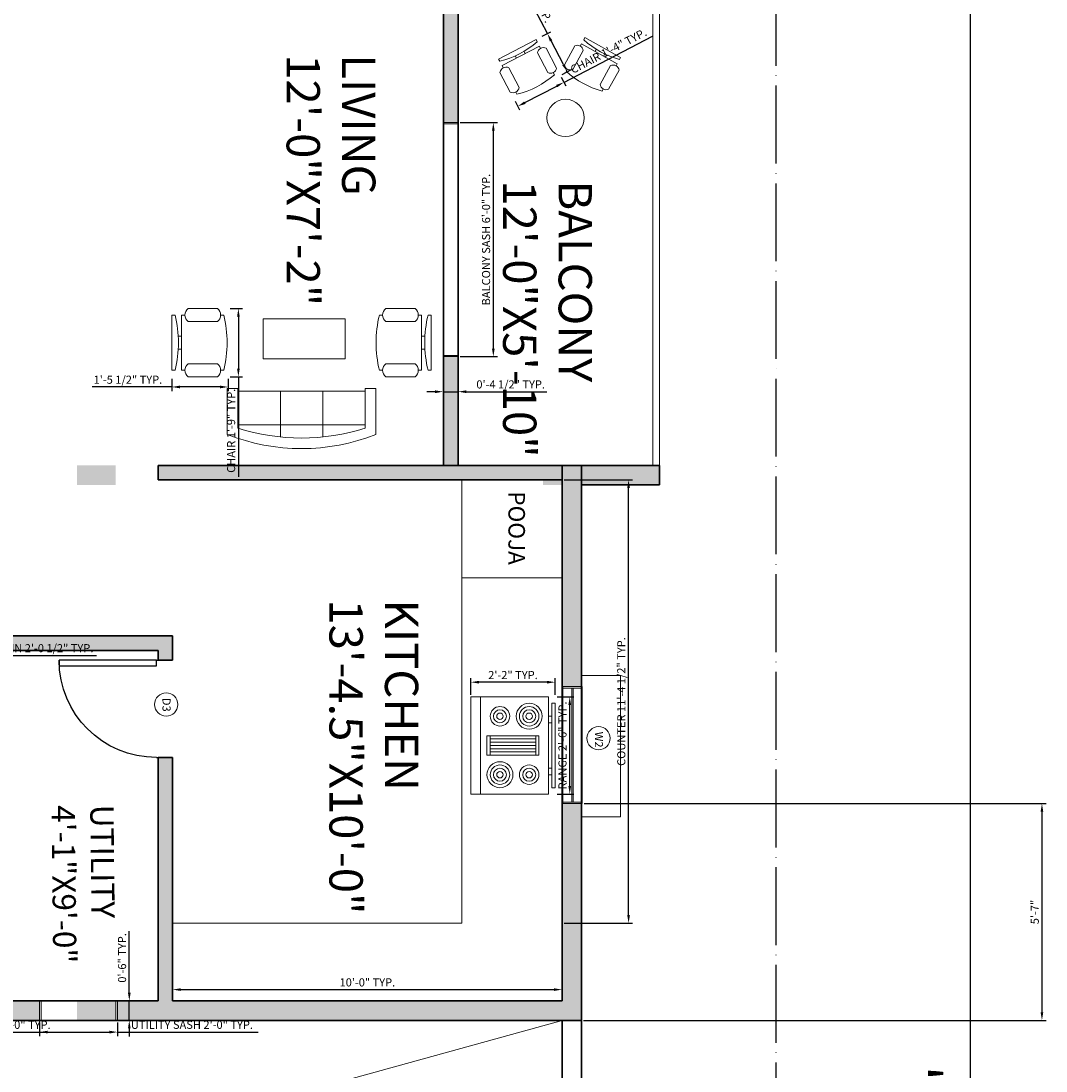
# Model space of a CAD drawing. Units: inches. Extents: x 7028582 to 7030319, y 63109697 to 63111305.
# Tile 16 of 18: x 7030003 to 7030319, y 63110530 to 63110853. Entities that reach past the tile are written whole.
import ezdxf

# ---------------------------------------------------------------- set-up
doc = ezdxf.new("R2010")
doc.units = ezdxf.units.IN
doc.linetypes.add('ACAD_ISO04W100', pattern=[30, 24, -3, 0, -3])
for name, color, linetype, lineweight in [('A-AREA-IDEN', 7, 'Continuous', 18), ('A-DOOR-IDEN', 20, 'Continuous', 13), ('A-EQPM', 9, 'Continuous', 18), ('A-FLOR-CASE', 9, 'Continuous', 18), ('A-FLOR-HRAL', 5, 'Continuous', 18), ('A-FLOR-OPEN', 7, 'Continuous', 13), ('A-GLAZ-IDEN', 20, 'Continuous', 13), ('A-WALL-PATT', 8, 'Continuous', 13), ('C-ANNO-DIMS', 7, 'Continuous', 18), ('C-PROP', 1, 'ACAD_ISO04W100', 25), ('doors', 20, 'Continuous', 25), ('furniture', 9, 'Continuous', 18), ('S-COLS-PATT', 220, 'Continuous', 100), ('walls', 6, 'Continuous', 35), ('WINDOW SHADOW', 9, 'Continuous', 13), ('windows', 5, 'Continuous', 18)]:
    doc.layers.add(name, color=color, linetype=linetype, lineweight=lineweight)
doc.styles.get("Standard").update_dxf_attribs({"font": 'arial.ttf'})
doc.dimstyles.new('ISO-25', dxfattribs={"dimtxt": 2.5, "dimasz": 2.5, "dimexe": 1.25, "dimexo": 0.625, "dimtad": 1, "dimlunit": 4, "dimtxsty": 'Standard', "dimcen": 2.5, "dimadec": 0, "dimazin": 0, "dimtfac": 1, "dimtmove": 0, "dimatfit": 3, "dimfxl": 1, "dimarcsym": 0})

# ---------------------------------------------------------------- blocks, each defined once
blk = doc.blocks.new('*U2')
for p, q in [((0, 0), (0, -5)), ((30, 0), (30, -5))]:
    blk.add_line(p, q)
blk.add_lwpolyline([(0, 0), (0, 30), (1.75, 30), (1.75, 0)], close=True)
blk.add_arc((0, 0), 30, 0, 90)
blk = doc.blocks.new('Range-Oven - 30 in top')
for p, q in [((0, -3), (30, -3)), ((12, -6), (18, -6)), ((13, -20), (13, -6)), ((14, -6), (14, -20)), ((15, -20), (15, -6)), ((16, -6), (16, -20)), ((17, -20), (17, -6)), ((18, -20), (12, -20)), ((6, -24), (6, -25)), ((8, -25), (8, -24)), ((22, -25), (22, -24)), ((24, -24), (24, -25))]:
    blk.add_line(p, q)
for points in [[(0, -24), (0, 0), (30, 0), (30, -24)], [(12, -21), (12, -5), (18, -5), (18, -21)], [(2, -26), (2, -25), (28, -25), (28, -26)]]:
    blk.add_lwpolyline(points, close=True)
for centre, radius in [((6, -9), 4), ((6, -9), 3), ((24, -9), 3), ((6, -9), 2), ((6, -9), 1), ((24, -9), 2), ((24, -9), 1), ((6, -18), 3), ((6, -18), 2), ((24, -18), 4), ((24, -18), 3), ((24, -18), 2), ((6, -18), 1), ((24, -18), 1)]:
    blk.add_circle(centre, radius)
blk = doc.blocks.new('Chair - Desk')
for p, q in [((-8.5, 0), (-8.5, -1)), ((-8.5, 0), (8.5, 0)), ((8.5, 0), (8.5, -1)), ((-8.5, -3), (-8.5, -4)), ((-8.5, -3), (8.5, -3)), ((-2, -3), (-2, -1.9355)), ((2, -1.9576), (2, -3)), ((8.5, -3), (8.5, -4)), ((-10.5, -5), (-10.5, -14)), ((-6.5, -14), (-6.5, -5)), ((6.5, -5), (6.5, -14)), ((10.5, -14), (10.5, -5)), ((-8.5, -15), (-8.5, -16)), ((8.5, -15), (8.5, -16))]:
    blk.add_line(p, q)
for centre, radius, start, end in [((0, 34.625), 36.625, 256.5803, 283.4197), ((-8.5, -6.5), 2.5, 36.8699, 143.1301), ((8.5, -6.5), 2.5, 36.8699, 143.1301), ((-8.5, -12.5), 2.5, 216.8699, 323.1301), ((0, 19.625), 36.625, 256.5803, 283.4197), ((8.5, -12.5), 2.5, 216.8699, 323.1301)]:
    blk.add_arc(centre, radius, start, end)
blk = doc.blocks.new('Sofa - Roundback 7 ft.')
for p, q in [((-36.000027, -34), (-36.000027, -11.4696)), ((-12.00002, -32.4421), (-12.00003, -6.5971)), ((11.99997, -32.4421), (11.99998, -6.5971)), ((35.99998, -34), (35.99998, -11.4696)), ((-35.999844, -13.3819), (35.9998, -13.3819)), ((-36.000027, -32.4421), (35.99998, -32.4421))]:
    blk.add_line(p, q)
for points in [[(-36.000027, -34), (-42.000027, -34), (-42.000027, -8)], [(41.99998, -8), (41.99998, -34), (35.99998, -34)]]:
    blk.add_lwpolyline(points)
for centre, radius, start, end in [((0, -114.25), 114.25, 68.43141, 111.5686), ((-0.00001, -127.1968), 121.1968, 72.72033, 107.2797)]:
    blk.add_arc(centre, radius, start, end)
blk = doc.blocks.new('*D10')
at = {"layer": 'C-ANNO-DIMS', "color": 0, "lineweight": -2, "transparency": 16777216}
for p, q in [((7030236.33, 63111093.06), (7030296.71, 63111093.06)), ((7030295.46, 63111090.56), (7030295.46, 63109909.06)), ((7030236.33, 63109906.56), (7030296.71, 63109906.56))]:
    blk.add_line(p, q, dxfattribs=at)
at = {"layer": 'C-ANNO-DIMS', "color": 0, "lineweight": 100, "transparency": 16777216}
for points in [[(7030295.04, 63111090.56), (7030295.88, 63111090.56), (7030295.46, 63111093.06)], [(7030295.04, 63109909.06), (7030295.88, 63109909.06), (7030295.46, 63109906.56)]]:
    blk.add_solid(points, dxfattribs=at)
at = {"layer": 'Defpoints', "color": 0, "lineweight": 100, "transparency": 16777216}
for p in [(7030235.71, 63111093.06), (7030235.71, 63109906.56), (7030295.46, 63109906.56)]:
    blk.add_point(p, dxfattribs=at)
at = {"layer": 'C-ANNO-DIMS', "color": 0, "transparency": 16777216, "insert": (7030280.69, 63110499.81), "char_height": 12, "attachment_point": 5, "rotation": 90}
blk.add_mtext('98\'-10{\\H1x;\\S1/2;}"', dxfattribs=at)
blk = doc.blocks.new('WIN-SASH-36')
for p, q in [((0, 36.05), (0, 0)), ((6, 0), (6, 36.05)), ((6, 35.55), (0, 35.55)), ((2.8, 35.55), (2.8, 0.5)), ((3.2, 35.55), (3.2, 0.5)), ((0, 0.5), (6, 0.5))]:
    blk.add_line(p, q)
blk = doc.blocks.new('WIN-SASH-24-FRAME')
for p, q in [((24.05, 6), (0, 6)), ((0.5, 6), (0.5, 0)), ((23.55, 0), (23.55, 6)), ((0, 0), (24.05, 0))]:
    blk.add_line(p, q)
blk = doc.blocks.new('WIN-SASH-BALCONY')
for p, q in [((0.13, 72.09), (0.13, 36.05)), ((4.63, 71.71), (0.13, 71.71)), ((4.63, 36.05), (4.63, 72.09)), ((0, 0.02), (0.13, 36.05)), ((0.13, 35.68), (0.13, 35.68)), ((4.63, 36.04), (4.5, 0)), ((4.5, 0.37), (0, 0.39))]:
    blk.add_line(p, q)
blk = doc.blocks.new('WINDOW-SHADE-SIDE-44')
for p, q in [((12, 43.55), (0, 43.55)), ((12, 0), (12, 43.55)), ((0, 0), (12, 0))]:
    blk.add_line(p, q)
blk = doc.blocks.new('KITCHEN-COUNTER')
for p, q in [((89.09, 136.54), (89.09, 16.65)), ((120, 106.35), (89.09, 106.35)), ((89.09, 16.65), (89.09, 0)), ((89.09, 0), (0, 0))]:
    blk.add_line(p, q)
blk = doc.blocks.new('BALCONY-GUARD-12FT')
for p, q in [((0, 144), (0, 0)), ((2, 144), (2, 0))]:
    blk.add_line(p, q)
blk = doc.blocks.new('TABLE-COFFEE-RECT')
blk.add_lwpolyline([(25.34, 12.34), (0, 12.34), (0, 0), (25.34, 0)], close=True)
blk = doc.blocks.new('TAG-D3-MT-R')
blk.add_circle((3.58, 3.58), 3.58)
at = {"insert": (4.93, 5.6), "char_height": 2.5, "attachment_point": 1, "rotation": 270}
blk.add_mtext_dynamic_manual_height_columns('D3', width=2.5021, gutter_width=12.5, heights=[0], dxfattribs=at)
blk = doc.blocks.new('TAG-W2-MT-R')
blk.add_circle((3.58, 3.58), 3.58)
at = {"insert": (4.93, 5.6), "char_height": 2.5, "attachment_point": 1, "rotation": 270}
blk.add_mtext_dynamic_manual_height_columns('W2', width=2.5021, gutter_width=12.5, heights=[0], dxfattribs=at)
blk = doc.blocks.new('TABLE-BALCONY-ROUND')
blk.add_circle((5.75, 5.75), 5.75)
blk = doc.blocks.new('*D49')
at = {"layer": 'C-ANNO-DIMS', "color": 0, "lineweight": -2, "transparency": 16777216}
for p, q in [((7030067.44, 63110764.87), (7030071.21, 63110764.87)), ((7030069.96, 63110762.37), (7030069.96, 63110746.37)), ((7030067.44, 63110743.87), (7030071.21, 63110743.87)), ((7030069.96, 63110743.87), (7030069.96, 63110713.07))]:
    blk.add_line(p, q, dxfattribs=at)
at = {"layer": 'C-ANNO-DIMS', "color": 0, "lineweight": 100, "transparency": 16777216}
for points in [[(7030069.55, 63110762.37), (7030070.38, 63110762.37), (7030069.96, 63110764.87)], [(7030069.55, 63110746.37), (7030070.38, 63110746.37), (7030069.96, 63110743.87)]]:
    blk.add_solid(points, dxfattribs=at)
at = {"layer": 'Defpoints', "color": 0, "lineweight": 100, "transparency": 16777216}
for p in [(7030066.81, 63110764.87), (7030066.81, 63110743.87), (7030069.96, 63110743.87)]:
    blk.add_point(p, dxfattribs=at)
at = {"layer": 'C-ANNO-DIMS', "color": 0, "transparency": 16777216, "insert": (7030068.05, 63110727.22), "char_height": 2.5, "attachment_point": 5, "rotation": 90}
blk.add_mtext('CHAIR 1\'-9" TYP.', dxfattribs=at)
blk = doc.blocks.new('*D50')
at = {"layer": 'C-ANNO-DIMS', "color": 0, "lineweight": -2, "transparency": 16777216}
for p, q in [((7030049.48, 63110740.72), (7030024.9, 63110740.72)), ((7030049.48, 63110743.24), (7030049.48, 63110739.47)), ((7030064.31, 63110740.72), (7030051.98, 63110740.72)), ((7030066.81, 63110743.24), (7030066.81, 63110739.47))]:
    blk.add_line(p, q, dxfattribs=at)
at = {"layer": 'C-ANNO-DIMS', "color": 0, "lineweight": 100, "transparency": 16777216}
for points in [[(7030051.98, 63110741.13), (7030051.98, 63110740.3), (7030049.48, 63110740.72)], [(7030064.31, 63110741.13), (7030064.31, 63110740.3), (7030066.81, 63110740.72)]]:
    blk.add_solid(points, dxfattribs=at)
at = {"layer": 'Defpoints', "color": 0, "lineweight": 100, "transparency": 16777216}
for p in [(7030049.48, 63110743.87), (7030066.81, 63110743.87), (7030049.48, 63110740.72)]:
    blk.add_point(p, dxfattribs=at)
at = {"layer": 'C-ANNO-DIMS', "color": 0, "transparency": 16777216, "insert": (7030035.94, 63110742.63), "char_height": 2.5, "attachment_point": 5}
blk.add_mtext('1\'-5 1/2" TYP.', dxfattribs=at)
blk = doc.blocks.new('*D53')
at = {"layer": 'C-ANNO-DIMS', "color": 0, "lineweight": -2, "transparency": 16777216}
for p, q in [((7030170.27, 63110834.58), (7030197.58, 63110848.82)), ((7030169.44, 63110836.16), (7030170.84, 63110833.48)), ((7030158.25, 63110828.32), (7030168.05, 63110833.43)), ((7030155.21, 63110828.75), (7030156.61, 63110826.06))]:
    blk.add_line(p, q, dxfattribs=at)
at = {"layer": 'C-ANNO-DIMS', "color": 0, "lineweight": 100, "transparency": 16777216}
for points in [[(7030167.86, 63110833.8), (7030168.24, 63110833.06), (7030170.27, 63110834.58)], [(7030158.06, 63110828.69), (7030158.44, 63110827.95), (7030156.03, 63110827.17)]]:
    blk.add_solid(points, dxfattribs=at)
at = {"layer": 'Defpoints', "color": 0, "lineweight": 100, "transparency": 16777216}
for p in [(7030169.15, 63110836.72), (7030170.27, 63110834.58), (7030154.92, 63110829.3)]:
    blk.add_point(p, dxfattribs=at)
at = {"layer": 'C-ANNO-DIMS', "color": 0, "transparency": 16777216, "insert": (7030184.14, 63110843.98), "char_height": 2.5, "attachment_point": 5, "rotation": 27.5292}
blk.add_mtext('CHAIR 1\'-4" TYP.', dxfattribs=at)
blk = doc.blocks.new('*D54')
at = {"layer": 'C-ANNO-DIMS', "color": 0, "lineweight": -2, "transparency": 16777216}
for p, q in [((7030165.17, 63110849.58), (7030156.5, 63110866.21)), ((7030163.58, 63110848.76), (7030166.27, 63110850.16)), ((7030170.13, 63110840.05), (7030166.32, 63110847.36)), ((7030169.71, 63110837.01), (7030172.4, 63110838.41))]:
    blk.add_line(p, q, dxfattribs=at)
at = {"layer": 'C-ANNO-DIMS', "color": 0, "lineweight": 100, "transparency": 16777216}
for points in [[(7030166.69, 63110847.56), (7030165.95, 63110847.17), (7030165.17, 63110849.58)], [(7030170.5, 63110840.24), (7030169.76, 63110839.86), (7030171.29, 63110837.83)]]:
    blk.add_solid(points, dxfattribs=at)
at = {"layer": 'Defpoints', "color": 0, "lineweight": 100, "transparency": 16777216}
for p in [(7030163.03, 63110848.47), (7030165.17, 63110849.58), (7030169.15, 63110836.72)]:
    blk.add_point(p, dxfattribs=at)
at = {"layer": 'C-ANNO-DIMS', "color": 0, "transparency": 16777216, "insert": (7030161.92, 63110859.87), "char_height": 2.5, "attachment_point": 5, "rotation": 297.5292}
blk.add_mtext('1\'-1" TYP.', dxfattribs=at)
blk = doc.blocks.new('*D55')
at = {"layer": 'C-ANNO-DIMS', "color": 0, "lineweight": -2, "transparency": 16777216}
for p, q in [((7029949.93, 63110544.93), (7029949.93, 63110540.7)), ((7029973.98, 63110544.93), (7029973.98, 63110540.7)), ((7029952.43, 63110541.95), (7029971.48, 63110541.95)), ((7029973.98, 63110541.95), (7030013.86, 63110541.95))]:
    blk.add_line(p, q, dxfattribs=at)
at = {"layer": 'C-ANNO-DIMS', "color": 0, "lineweight": 100, "transparency": 16777216}
for points in [[(7029952.43, 63110542.37), (7029952.43, 63110541.53), (7029949.93, 63110541.95)], [(7029971.48, 63110542.37), (7029971.48, 63110541.53), (7029973.98, 63110541.95)]]:
    blk.add_solid(points, dxfattribs=at)
at = {"layer": 'Defpoints', "color": 0, "lineweight": 100, "transparency": 16777216}
for p in [(7029949.93, 63110545.56), (7029973.98, 63110545.56), (7029973.98, 63110541.95)]:
    blk.add_point(p, dxfattribs=at)
at = {"layer": 'C-ANNO-DIMS', "color": 0, "transparency": 16777216, "insert": (7029995.17, 63110543.87), "char_height": 2.5, "attachment_point": 5}
blk.add_mtext('VENT SASH 2\'-0" TYP.', dxfattribs=at)
blk = doc.blocks.new('*D61')
at = {"layer": 'C-ANNO-DIMS', "color": 0, "lineweight": -2, "transparency": 16777216}
for p, q in [((7029965.55, 63110654.94), (7029965.55, 63110659.24)), ((7029968.05, 63110657.99), (7029987.6, 63110657.99)), ((7029990.1, 63110654.94), (7029990.1, 63110659.24)), ((7029990.1, 63110657.99), (7030026.26, 63110657.99))]:
    blk.add_line(p, q, dxfattribs=at)
at = {"layer": 'C-ANNO-DIMS', "color": 0, "lineweight": 100, "transparency": 16777216}
for points in [[(7029968.05, 63110658.41), (7029968.05, 63110657.58), (7029965.55, 63110657.99)], [(7029987.6, 63110658.41), (7029987.6, 63110657.58), (7029990.1, 63110657.99)]]:
    blk.add_solid(points, dxfattribs=at)
at = {"layer": 'Defpoints', "color": 0, "lineweight": 100, "transparency": 16777216}
for p in [(7029990.1, 63110657.99), (7029965.55, 63110654.31), (7029990.1, 63110654.31)]:
    blk.add_point(p, dxfattribs=at)
at = {"layer": 'C-ANNO-DIMS', "color": 0, "transparency": 16777216, "insert": (7030009.43, 63110659.91), "char_height": 2.5, "attachment_point": 5}
blk.add_mtext('BASIN 2\'-0 1/2" TYP.', dxfattribs=at)
blk = doc.blocks.new('*D75')
at = {"layer": 'C-ANNO-DIMS', "color": 0, "lineweight": -2, "transparency": 16777216}
for p, q in [((7030168.19, 63110645.26), (7030173.32, 63110645.26)), ((7030172.07, 63110617.76), (7030172.07, 63110642.76)), ((7030168.19, 63110615.26), (7030173.32, 63110615.26))]:
    blk.add_line(p, q, dxfattribs=at)
at = {"layer": 'C-ANNO-DIMS', "color": 0, "lineweight": 100, "transparency": 16777216}
for points in [[(7030171.65, 63110642.76), (7030172.48, 63110642.76), (7030172.07, 63110645.26)], [(7030171.65, 63110617.76), (7030172.48, 63110617.76), (7030172.07, 63110615.26)]]:
    blk.add_solid(points, dxfattribs=at)
at = {"layer": 'Defpoints', "color": 0, "lineweight": 100, "transparency": 16777216}
for p in [(7030167.57, 63110645.26), (7030172.07, 63110645.26), (7030167.57, 63110615.26)]:
    blk.add_point(p, dxfattribs=at)
at = {"layer": 'C-ANNO-DIMS', "color": 0, "transparency": 16777216, "insert": (7030170.15, 63110630.26), "char_height": 2.5, "attachment_point": 5, "rotation": 90}
blk.add_mtext('RANGE 2\'-6" TYP.', dxfattribs=at)
blk = doc.blocks.new('*D76')
at = {"layer": 'C-ANNO-DIMS', "color": 0, "lineweight": -2, "transparency": 16777216}
for p, q in [((7030141.57, 63110645.88), (7030141.57, 63110651.01)), ((7030167.57, 63110645.88), (7030167.57, 63110651.01)), ((7030165.07, 63110649.76), (7030144.07, 63110649.76))]:
    blk.add_line(p, q, dxfattribs=at)
at = {"layer": 'C-ANNO-DIMS', "color": 0, "lineweight": 100, "transparency": 16777216}
for points in [[(7030144.07, 63110650.17), (7030144.07, 63110649.34), (7030141.57, 63110649.76)], [(7030165.07, 63110650.17), (7030165.07, 63110649.34), (7030167.57, 63110649.76)]]:
    blk.add_solid(points, dxfattribs=at)
at = {"layer": 'Defpoints', "color": 0, "lineweight": 100, "transparency": 16777216}
for p in [(7030141.57, 63110649.76), (7030141.57, 63110645.26), (7030167.57, 63110645.26)]:
    blk.add_point(p, dxfattribs=at)
at = {"layer": 'C-ANNO-DIMS', "color": 0, "transparency": 16777216, "insert": (7030154.57, 63110651.64), "char_height": 2.5, "attachment_point": 5}
blk.add_mtext('2\'-2" TYP.', dxfattribs=at)
blk = doc.blocks.new('*D79')
at = {"layer": 'C-ANNO-DIMS', "color": 0, "lineweight": -2, "transparency": 16777216}
for p, q in [((7030008.7, 63110544.93), (7030008.7, 63110540.7)), ((7030032.75, 63110544.93), (7030032.75, 63110540.7)), ((7030011.2, 63110541.95), (7030030.25, 63110541.95)), ((7030032.75, 63110541.95), (7030076.06, 63110541.95))]:
    blk.add_line(p, q, dxfattribs=at)
at = {"layer": 'C-ANNO-DIMS', "color": 0, "lineweight": 100, "transparency": 16777216}
for points in [[(7030011.2, 63110542.37), (7030011.2, 63110541.53), (7030008.7, 63110541.95)], [(7030030.25, 63110542.37), (7030030.25, 63110541.53), (7030032.75, 63110541.95)]]:
    blk.add_solid(points, dxfattribs=at)
at = {"layer": 'Defpoints', "color": 0, "lineweight": 100, "transparency": 16777216}
for p in [(7030008.7, 63110545.56), (7030032.75, 63110545.56), (7030032.75, 63110541.95)]:
    blk.add_point(p, dxfattribs=at)
at = {"layer": 'C-ANNO-DIMS', "color": 0, "transparency": 16777216, "insert": (7030055.65, 63110543.87), "char_height": 2.5, "attachment_point": 5}
blk.add_mtext('UTILITY SASH 2\'-0" TYP.', dxfattribs=at)
blk = doc.blocks.new('*D80')
at = {"layer": 'C-ANNO-DIMS', "color": 0, "lineweight": -2, "transparency": 16777216}
for p, q in [((7030036.35, 63110554.06), (7030036.35, 63110573.05)), ((7030033.37, 63110551.56), (7030037.6, 63110551.56)), ((7030036.35, 63110545.56), (7030036.35, 63110551.56)), ((7030033.37, 63110545.56), (7030037.6, 63110545.56)), ((7030036.35, 63110543.06), (7030036.35, 63110540.56))]:
    blk.add_line(p, q, dxfattribs=at)
at = {"layer": 'C-ANNO-DIMS', "color": 0, "lineweight": 100, "transparency": 16777216}
for points in [[(7030035.94, 63110554.06), (7030036.77, 63110554.06), (7030036.35, 63110551.56)], [(7030035.94, 63110543.06), (7030036.77, 63110543.06), (7030036.35, 63110545.56)]]:
    blk.add_solid(points, dxfattribs=at)
at = {"layer": 'Defpoints', "color": 0, "lineweight": 100, "transparency": 16777216}
for p in [(7030032.75, 63110551.56), (7030036.35, 63110551.56), (7030032.75, 63110545.56)]:
    blk.add_point(p, dxfattribs=at)
at = {"layer": 'C-ANNO-DIMS', "color": 0, "transparency": 16777216, "insert": (7030034.45, 63110564.8), "char_height": 2.5, "attachment_point": 5, "rotation": 90}
blk.add_mtext('0\'-6" TYP.', dxfattribs=at)
blk = doc.blocks.new('*D81')
at = {"layer": 'C-ANNO-DIMS', "color": 0, "lineweight": -2, "transparency": 16777216}
for p, q in [((7030138.33, 63110822.16), (7030149.77, 63110822.16)), ((7030148.52, 63110752.57), (7030148.52, 63110819.66)), ((7030138.33, 63110750.07), (7030149.77, 63110750.07))]:
    blk.add_line(p, q, dxfattribs=at)
at = {"layer": 'C-ANNO-DIMS', "color": 0, "lineweight": 100, "transparency": 16777216}
for points in [[(7030148.1, 63110819.66), (7030148.94, 63110819.66), (7030148.52, 63110822.16)], [(7030148.1, 63110752.57), (7030148.94, 63110752.57), (7030148.52, 63110750.07)]]:
    blk.add_solid(points, dxfattribs=at)
at = {"layer": 'Defpoints', "color": 0, "lineweight": 100, "transparency": 16777216}
for p in [(7030137.71, 63110822.16), (7030148.52, 63110822.16), (7030137.71, 63110750.07)]:
    blk.add_point(p, dxfattribs=at)
at = {"layer": 'C-ANNO-DIMS', "color": 0, "transparency": 16777216, "insert": (7030146.6, 63110786.12), "char_height": 2.5, "attachment_point": 5, "rotation": 90}
blk.add_mtext('BALCONY SASH 6\'-0" TYP.', dxfattribs=at)
blk = doc.blocks.new('*D82')
at = {"layer": 'C-ANNO-DIMS', "color": 0, "lineweight": -2, "transparency": 16777216}
for p, q in [((7030133.08, 63110749.45), (7030133.08, 63110738.01)), ((7030137.71, 63110749.45), (7030137.71, 63110738.01)), ((7030130.58, 63110739.26), (7030128.08, 63110739.26)), ((7030133.08, 63110739.26), (7030137.71, 63110739.26)), ((7030140.21, 63110739.26), (7030165.02, 63110739.26))]:
    blk.add_line(p, q, dxfattribs=at)
at = {"layer": 'C-ANNO-DIMS', "color": 0, "lineweight": 100, "transparency": 16777216}
for points in [[(7030130.58, 63110739.68), (7030130.58, 63110738.84), (7030133.08, 63110739.26)], [(7030140.21, 63110739.68), (7030140.21, 63110738.84), (7030137.71, 63110739.26)]]:
    blk.add_solid(points, dxfattribs=at)
at = {"layer": 'Defpoints', "color": 0, "lineweight": 100, "transparency": 16777216}
for p in [(7030133.08, 63110750.07), (7030137.71, 63110750.07), (7030137.71, 63110739.26)]:
    blk.add_point(p, dxfattribs=at)
at = {"layer": 'C-ANNO-DIMS', "color": 0, "transparency": 16777216, "insert": (7030153.86, 63110741.18), "char_height": 2.5, "attachment_point": 5}
blk.add_mtext('0\'-4 1/2" TYP.', dxfattribs=at)
blk = doc.blocks.new('*D85')
at = {"layer": 'C-ANNO-DIMS', "color": 0, "lineweight": -2, "transparency": 16777216}
for p, q in [((7030170.33, 63110712.06), (7030191.44, 63110712.06)), ((7030190.19, 63110578.02), (7030190.19, 63110709.56)), ((7030170.33, 63110575.52), (7030191.44, 63110575.52))]:
    blk.add_line(p, q, dxfattribs=at)
at = {"layer": 'C-ANNO-DIMS', "color": 0, "lineweight": 100, "transparency": 16777216}
for points in [[(7030189.77, 63110709.56), (7030190.6, 63110709.56), (7030190.19, 63110712.06)], [(7030189.77, 63110578.02), (7030190.6, 63110578.02), (7030190.19, 63110575.52)]]:
    blk.add_solid(points, dxfattribs=at)
at = {"layer": 'Defpoints', "color": 0, "lineweight": 100, "transparency": 16777216}
for p in [(7030169.71, 63110712.06), (7030190.19, 63110712.06), (7030169.71, 63110575.52)]:
    blk.add_point(p, dxfattribs=at)
at = {"layer": 'C-ANNO-DIMS', "color": 0, "transparency": 16777216, "insert": (7030188.27, 63110643.79), "char_height": 2.5, "attachment_point": 5, "rotation": 90}
blk.add_mtext('COUNTER 11\'-4 1/2" TYP.', dxfattribs=at)
blk = doc.blocks.new('*D86')
at = {"layer": 'C-ANNO-DIMS', "color": 0, "lineweight": -2, "transparency": 16777216}
for p, q in [((7030049.71, 63110574.89), (7030049.71, 63110553.79)), ((7030169.71, 63110574.89), (7030169.71, 63110553.79)), ((7030052.21, 63110555.04), (7030167.21, 63110555.04))]:
    blk.add_line(p, q, dxfattribs=at)
at = {"layer": 'C-ANNO-DIMS', "color": 0, "lineweight": 100, "transparency": 16777216}
for points in [[(7030052.21, 63110555.45), (7030052.21, 63110554.62), (7030049.71, 63110555.04)], [(7030167.21, 63110555.45), (7030167.21, 63110554.62), (7030169.71, 63110555.04)]]:
    blk.add_solid(points, dxfattribs=at)
at = {"layer": 'Defpoints', "color": 0, "lineweight": 100, "transparency": 16777216}
for p in [(7030049.71, 63110575.52), (7030169.71, 63110575.52), (7030169.71, 63110555.04)]:
    blk.add_point(p, dxfattribs=at)
at = {"layer": 'C-ANNO-DIMS', "color": 0, "transparency": 16777216, "insert": (7030109.71, 63110556.94), "char_height": 2.5, "attachment_point": 5}
blk.add_mtext('10\'-0" TYP.', dxfattribs=at)
blk = doc.blocks.new('*D118')
at = {"layer": 'C-ANNO-DIMS', "color": 0, "lineweight": -2, "transparency": 16777216}
for p, q in [((7030176.52, 63110612.34), (7030318.81, 63110612.34)), ((7030317.56, 63110609.84), (7030317.56, 63110548.06)), ((7030176.33, 63110545.56), (7030318.81, 63110545.56))]:
    blk.add_line(p, q, dxfattribs=at)
at = {"layer": 'C-ANNO-DIMS', "color": 0, "lineweight": 100, "transparency": 16777216}
for points in [[(7030317.14, 63110609.84), (7030317.97, 63110609.84), (7030317.56, 63110612.34)], [(7030317.14, 63110548.06), (7030317.97, 63110548.06), (7030317.56, 63110545.56)]]:
    blk.add_solid(points, dxfattribs=at)
at = {"layer": 'Defpoints', "color": 0, "lineweight": 100, "transparency": 16777216}
for p in [(7030175.9, 63110612.34), (7030175.71, 63110545.56), (7030317.56, 63110545.56)]:
    blk.add_point(p, dxfattribs=at)
at = {"layer": 'C-ANNO-DIMS', "color": 0, "transparency": 16777216, "insert": (7030315.66, 63110578.95), "char_height": 2.5, "attachment_point": 5, "rotation": 90}
blk.add_mtext('5\'-7"', dxfattribs=at)

msp = doc.modelspace()

# ---------------------------------------------------------------- hatches: boundary and pattern name
at = {"layer": 'A-WALL-PATT'}
h = msp.add_hatch(color=256, dxfattribs=at)
h.dxf.hatch_style = 1
h.paths.add_polyline_path([(7030137.705, 63110860.557), (7030133.205, 63110860.557), (7030133.205, 63110822.163), (7030137.705, 63110822.163)])
h = msp.add_hatch(color=256, dxfattribs=at)
h.dxf.hatch_style = 1
h.paths.add_polyline_path([(7030137.705, 63110750.074), (7030133.205, 63110750.09), (7030133.205, 63110716.557), (7030137.705, 63110716.557)])
h = msp.add_hatch(color=256, dxfattribs=at)
h.dxf.hatch_style = 1
h.paths.add_polyline_path([(7030169.705, 63110716.557), (7030045.205, 63110716.557), (7030045.205, 63110712.057), (7030169.705, 63110712.057)])
h = msp.add_hatch(color=256, dxfattribs=at)
h.dxf.hatch_style = 1
h.paths.add_polyline_path([(7030175.705, 63110716.557), (7030169.705, 63110716.557), (7030169.705, 63110648.386), (7030175.705, 63110648.386)])
h = msp.add_hatch(color=256, dxfattribs=at)
h.dxf.hatch_style = 1
h.paths.add_polyline_path([(7030199.705, 63110716.557), (7030175.705, 63110716.557), (7030175.705, 63110710.557), (7030199.705, 63110710.557)])
h = msp.add_hatch(color=256, dxfattribs=at)
h.dxf.hatch_style = 1
h.paths.add_polyline_path([(7030049.705, 63110664.057), (7029996.205, 63110664.057), (7029996.205, 63110659.557), (7030045.205, 63110659.557), (7030045.205, 63110656.557), (7030049.705, 63110656.557)])
h = msp.add_hatch(color=256, dxfattribs=at)
h.dxf.hatch_style = 1
h.paths.add_polyline_path([(7029996.205, 63110659.557), (7029991.705, 63110659.557), (7029991.705, 63110551.557), (7029973.979, 63110551.557), (7029973.979, 63110545.557), (7030008.697, 63110545.557), (7030008.697, 63110551.557), (7029996.205, 63110551.557)])
h = msp.add_hatch(color=256, dxfattribs=at)
h.dxf.hatch_style = 1
h.paths.add_polyline_path([(7030175.705, 63110612.338), (7030169.705, 63110612.338), (7030169.705, 63110551.557), (7030049.705, 63110551.557), (7030049.705, 63110626.557), (7030045.205, 63110626.557), (7030045.205, 63110551.557), (7030032.745, 63110551.557), (7030032.745, 63110545.557), (7030175.705, 63110545.557)])
at = {"layer": 'S-COLS-PATT'}
h = msp.add_hatch(color=256, dxfattribs=at)
h.dxf.hatch_style = 1
h.paths.add_polyline_path([(7030032.194, 63110716.557), (7030020.279, 63110716.557), (7030020.279, 63110710.557), (7030032.194, 63110710.557)])
h = msp.add_hatch(color=256, dxfattribs=at)
h.dxf.hatch_style = 1
h.paths.add_polyline_path([(7030175.705, 63110716.557), (7030163.791, 63110716.557), (7030163.791, 63110710.557), (7030175.705, 63110710.557)])
h = msp.add_hatch(color=256, dxfattribs=at)
h.dxf.hatch_style = 1
h.paths.add_polyline_path([(7030032.194, 63110551.607), (7030020.279, 63110551.607), (7030020.279, 63110545.607), (7030032.194, 63110545.607)])
h = msp.add_hatch(color=256, dxfattribs=at)
h.dxf.hatch_style = 1
h.paths.add_polyline_path([(7030175.705, 63110551.607), (7030163.791, 63110551.607), (7030163.791, 63110545.607), (7030175.705, 63110545.607)])

# ---------------------------------------------------------------- linework, layer by layer
at = {"layer": 'A-FLOR-OPEN'}
msp.add_line((7029838.205, 63110454.057), (7030169.705, 63110545.557), dxfattribs=at)
at = {"layer": 'C-PROP'}
msp.add_line((7030235.705, 63109906.557), (7030235.705, 63111093.057), dxfattribs=at)
at = {"layer": 'walls'}
for p, q in [((7030133.205, 63110860.557), (7030133.205, 63110716.557)), ((7030137.705, 63110860.557), (7030137.705, 63110716.557)), ((7030175.705, 63110716.557), (7030045.205, 63110716.557)), ((7030045.205, 63110712.057), (7030045.205, 63110716.557)), ((7030169.705, 63110551.557), (7030169.705, 63110716.557)), ((7030199.705, 63110716.557), (7030175.705, 63110716.557)), ((7030175.705, 63110281.557), (7030175.705, 63110716.557)), ((7030199.705, 63110710.557), (7030199.705, 63110716.557)), ((7030169.705, 63110712.057), (7030045.205, 63110712.057)), ((7030175.705, 63110710.557), (7030199.705, 63110710.557)), ((7030049.705, 63110664.057), (7029964.705, 63110664.057)), ((7030049.705, 63110656.557), (7030049.705, 63110664.057)), ((7030045.205, 63110659.557), (7029964.705, 63110659.557)), ((7030045.205, 63110659.557), (7030045.205, 63110656.557)), ((7030045.205, 63110656.557), (7030045.205, 63110659.557)), ((7030045.205, 63110656.557), (7030049.705, 63110656.557)), ((7030045.205, 63110551.557), (7030045.205, 63110626.557)), ((7030049.705, 63110626.557), (7030045.205, 63110626.557)), ((7030049.705, 63110551.557), (7030049.705, 63110626.557)), ((7030045.205, 63110551.557), (7029996.205, 63110551.557)), ((7030169.705, 63110551.557), (7030049.705, 63110551.557)), ((7030175.705, 63110545.557), (7029748.205, 63110545.557)), ((7030169.705, 63110281.557), (7030169.705, 63110545.557))]:
    msp.add_line(p, q, dxfattribs=at)
at = {"layer": 'windows'}
for p, q in [((7030137.705, 63110822.163), (7030133.205, 63110822.163)), ((7030137.577, 63110750.074), (7030133.077, 63110750.09)), ((7030175.898, 63110648.386), (7030169.898, 63110648.386)), ((7030169.898, 63110612.338), (7030175.898, 63110612.338)), ((7030008.697, 63110551.557), (7030008.697, 63110545.557)), ((7030032.745, 63110545.557), (7030032.745, 63110551.557))]:
    msp.add_line(p, q, dxfattribs=at)

# ---------------------------------------------------------------- block references
at = {"layer": 'A-DOOR-IDEN'}
msp.add_blockref('TAG-D3-MT-R', (7030044.153, 63110639.309), dxfattribs=at)
at = {"layer": 'A-EQPM', "rotation": 90}
msp.add_blockref('Range-Oven - 30 in top', (7030141.566, 63110615.257), dxfattribs=at)
at = {"layer": 'A-FLOR-CASE'}
msp.add_blockref('KITCHEN-COUNTER', (7030049.705, 63110575.518), dxfattribs=at)
at = {"layer": 'A-FLOR-HRAL'}
msp.add_blockref('BALCONY-GUARD-12FT', (7030197.705, 63110716.557), dxfattribs=at)
at = {"layer": 'A-GLAZ-IDEN'}
msp.add_blockref('TAG-W2-MT-R', (7030177.373, 63110628.907), dxfattribs=at)
at = {"layer": 'doors', "xscale": -1, "rotation": 90}
msp.add_blockref('*U2', (7030044.705, 63110656.557), dxfattribs=at)
at = {"layer": 'furniture'}
for name, p, xscale, yscale, zscale, rotation in [('Chair - Desk', (7030155.914, 63110844.758), 0.7643373636972337, 0.7643373636972337, 0.7643373636972337, 27.52919134002635), ('Chair - Desk', (7030182.234, 63110845.309), 0.740937522274531, 0.740937522274531, 0.740937522274531, 331.1002874626102), ('Sofa - Roundback 7 ft.', (7030089.438, 63110721.72), 0.5455524879488546, 0.5455524879488546, 0.5455524879488546, 180)]:
    msp.add_blockref(name, p, dxfattribs=dict(at, xscale=xscale, yscale=yscale, zscale=zscale, rotation=rotation))
for name, p in [('TABLE-BALCONY-ROUND', (7030165.023, 63110817.874)), ('TABLE-COFFEE-RECT', (7030077.552, 63110749.363))]:
    msp.add_blockref(name, p, dxfattribs=at)
at = {"layer": 'furniture', "xscale": -1, "rotation": 90}
msp.add_blockref('Chair - Desk', (7030049.481, 63110754.367), dxfattribs=at)
at = {"layer": 'furniture', "rotation": 270}
msp.add_blockref('Chair - Desk', (7030129.395, 63110754.367), dxfattribs=at)
at = {"layer": 'WINDOW SHADOW'}
msp.add_blockref('WINDOW-SHADE-SIDE-44', (7030175.705, 63110608.281), dxfattribs=at)
at = {"layer": 'windows'}
for name, p in [('WIN-SASH-BALCONY', (7030133.077, 63110750.074)), ('WIN-SASH-24-FRAME', (7030008.697, 63110545.557))]:
    msp.add_blockref(name, p, dxfattribs=at)
at = {"layer": 'windows', "rotation": 180}
msp.add_blockref('WIN-SASH-36', (7030175.898, 63110648.386), dxfattribs=at)

# ---------------------------------------------------------------- texts
at = {"layer": 'A-AREA-IDEN', "attachment_point": 1}
for s, width, gutter_width, insert, char_height, rotation in [('LIVING\\P12\'-0"X7\'-2"', 82.04322, 51.315, (7030112.192, 63110843.231), 10.26307, 270), ('BALCONY\\P12\'-0"X5\'-10"', 82.04322, 51.315, (7030178.895, 63110804.354), 10.26307, 270), ('POOJA', 15.69653, 25.463, (7030158.26, 63110708.57), 5.0926, 270), ('KITCHEN\\P13\'-4.5"X10\'-0"', 82.04322, 51.315, (7030125.386, 63110675.255), 10.26307, 270), ('UTILITY\\P4\'-1"X9\'-0"', 42.97461, 35.821, (7030031.482, 63110612.048), 7.16426, 270.6464)]:
    msp.add_mtext_dynamic_manual_height_columns(s, width=width, gutter_width=gutter_width, heights=[0], dxfattribs=dict(at, insert=insert, char_height=char_height, rotation=rotation))

# ---------------------------------------------------------------- dimensions: what is measured, and where the dimension line sits
at = {"layer": 'C-ANNO-DIMS'}
for base, p1, p2, override, picture, middle in [((7030295.462, 63109906.557), (7030235.705, 63111093.057), (7030235.705, 63109906.557), {"dimtxt": 12, "dimclrd": 0, "dimclre": 0, "dimclrt": 0}, '*D10', (7030280.685, 63110499.807)), ((7030317.555, 63110545.557), (7030175.898, 63110612.338), (7030175.705, 63110545.557), {"dimdec": 1, "dimlfac": 1, "dimrnd": 0, "dimzin": 1, "dimdsep": 46, "dimlunit": 4, "dimfrac": 2}, '*D118', (7030315.659, 63110578.947))]:
    dim = msp.add_linear_dim(base=base, p1=p1, p2=p2, angle=90, dimstyle='ISO-25', override=override, dxfattribs=at)
    dim.commit()
    dim.dimension.update_dxf_attribs({"geometry": picture, "text_midpoint": middle})
for base, p1, p2, angle, text, picture, middle in [((7030165.166, 63110849.58), (7030169.154, 63110836.719), (7030163.03, 63110848.468), 117.52919, '<> TYP.', '*D54', (7030161.922, 63110859.873)), ((7030170.267, 63110834.584), (7030154.92, 63110829.3), (7030169.154, 63110836.719), 27.52919, 'CHAIR <> TYP.', '*D53', (7030184.144, 63110843.979)), ((7030148.519, 63110822.163), (7030137.705, 63110750.074), (7030137.705, 63110822.163), 90, 'BALCONY SASH <> TYP.', '*D81', (7030146.6, 63110786.119)), ((7030069.965, 63110743.867), (7030066.815, 63110764.867), (7030066.815, 63110743.867), 270, 'CHAIR <> TYP.', '*D49', (7030068.047, 63110727.219)), ((7030049.481, 63110740.717), (7030066.815, 63110743.867), (7030049.481, 63110743.867), 180, '<> TYP.', '*D50', (7030035.942, 63110742.635)), ((7030190.186, 63110712.057), (7030169.705, 63110575.518), (7030169.705, 63110712.057), 90, 'COUNTER <> TYP.', '*D85', (7030188.268, 63110643.788)), ((7030141.566, 63110649.757), (7030167.566, 63110645.257), (7030141.566, 63110645.257), 180, '<> TYP.', '*D76', (7030154.566, 63110651.638)), ((7030172.066, 63110645.257), (7030167.566, 63110615.257), (7030167.566, 63110645.257), 90, 'RANGE <> TYP.', '*D75', (7030170.149, 63110630.257)), ((7030036.352, 63110551.557), (7030032.745, 63110545.557), (7030032.745, 63110551.557), 90, '<> TYP.', '*D80', (7030034.451, 63110564.801))]:
    dim = msp.add_linear_dim(base=base, p1=p1, p2=p2, angle=angle, text=text, dimstyle='ISO-25', override={"dimdec": 1, "dimlfac": 1, "dimrnd": 0, "dimzin": 1, "dimdsep": 46, "dimlunit": 4, "dimfrac": 2}, dxfattribs=at)
    dim.commit()
    dim.dimension.update_dxf_attribs({"geometry": picture, "text_midpoint": middle})
for base, p1, p2, text, picture, middle in [((7030137.705, 63110739.261), (7030133.077, 63110750.074), (7030137.705, 63110750.074), '<> TYP.', '*D82', (7030153.862, 63110741.179)), ((7029990.104, 63110657.993), (7029965.553, 63110654.311), (7029990.104, 63110654.311), 'BASIN <> TYP.', '*D61', (7030009.432, 63110659.911)), ((7030169.705, 63110555.038), (7030049.705, 63110575.518), (7030169.705, 63110575.518), '<> TYP.', '*D86', (7030109.705, 63110556.939)), ((7029973.979, 63110541.949), (7029949.931, 63110545.557), (7029973.979, 63110545.557), 'VENT SASH <> TYP.', '*D55', (7029995.171, 63110543.867)), ((7030032.745, 63110541.949), (7030008.697, 63110545.557), (7030032.745, 63110545.557), 'UTILITY SASH <> TYP.', '*D79', (7030055.651, 63110543.867))]:
    dim = msp.add_linear_dim(base=base, p1=p1, p2=p2, text=text, dimstyle='ISO-25', override={"dimdec": 1, "dimlfac": 1, "dimrnd": 0, "dimzin": 1, "dimdsep": 46, "dimlunit": 4, "dimfrac": 2}, dxfattribs=at)
    dim.commit()
    dim.dimension.update_dxf_attribs({"geometry": picture, "text_midpoint": middle})

doc.saveas('drawing.dxf')
